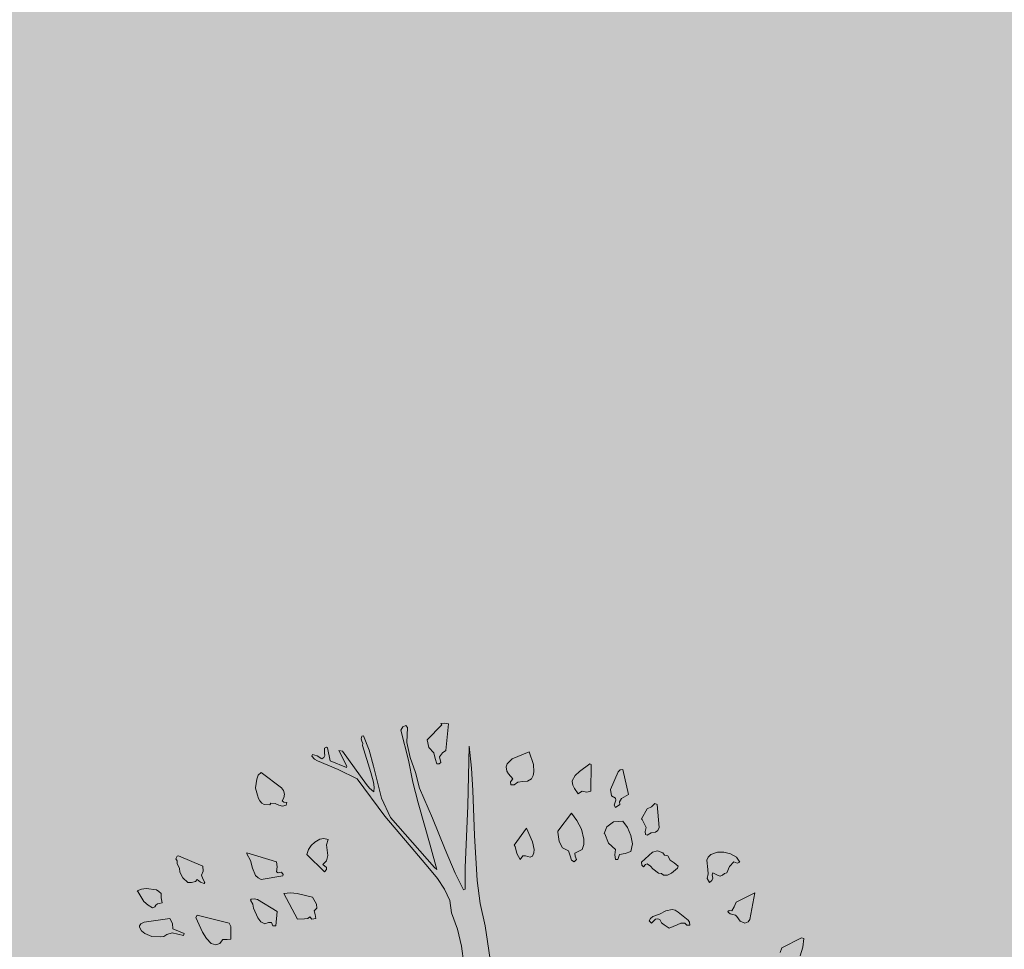
# Model space of a CAD drawing. Units: inches. Extents: x 84 to 1044, y -280 to 906.
# Tile 36 of 105: x 848 to 876, y -93 to -66. Entities that reach past the tile are written whole.
import ezdxf

# ---------------------------------------------------------------- set-up
doc = ezdxf.new("R2010")
doc.units = ezdxf.units.IN
doc.layers.add('L-PLNT', color=114, linetype='Continuous', lineweight=15)
doc.layers.add('L-PLNT-PATT', color=9, linetype='Continuous', lineweight=9, true_color=0xafd9aa)

# ---------------------------------------------------------------- blocks, each defined once
blk = doc.blocks.new('A$C37E508DF')
for p, q in [((0.6329, 1.5111), (0.6367, 1.5175)), ((0.6367, 1.5175), (0.6423, 1.5201)), ((0.6423, 1.5201), (0.6453, 1.5158)), ((0.6826, 1.493), (0.7096, 1.5209)), ((0.7083, 1.5239), (0.7152, 1.5244)), ((0.7096, 1.5209), (0.7083, 1.5239)), ((0.7152, 1.5244), (0.7225, 1.5231)), ((0.7225, 1.5231), (0.7174, 1.4729)), ((0.5583, 1.4948), (0.5596, 1.4995)), ((0.5596, 1.4995), (0.563, 1.5003)), ((0.563, 1.5003), (0.5737, 1.4733)), ((0.6475, 1.4545), (0.6329, 1.5111)), ((0.6453, 1.5158), (0.644, 1.4879)), ((0.5596, 1.4905), (0.5583, 1.4948)), ((0.5613, 1.4862), (0.5596, 1.4905)), ((0.5608, 1.4823), (0.5613, 1.4862)), ((0.5767, 1.4317), (0.5608, 1.4823)), ((0.644, 1.4879), (0.6505, 1.46)), ((0.6852, 1.4785), (0.6826, 1.493)), ((0.7589, 1.3691), (0.7615, 1.481)), ((0.7615, 1.481), (0.7658, 1.4395)), ((0.4657, 1.4622), (0.4669, 1.4652)), ((0.4708, 1.4566), (0.4657, 1.4622)), ((0.4669, 1.4652), (0.4755, 1.463)), ((0.4755, 1.463), (0.4845, 1.4575)), ((0.4884, 1.4596), (0.4905, 1.4635)), ((0.4897, 1.4772), (0.4935, 1.4789)), ((0.4897, 1.4678), (0.4897, 1.4772)), ((0.4905, 1.4635), (0.4897, 1.4678)), ((0.4935, 1.4789), (0.4952, 1.478)), ((0.4952, 1.478), (0.5004, 1.4532)), ((0.5313, 1.4437), (0.5167, 1.4729)), ((0.5167, 1.4729), (0.5231, 1.4716)), ((0.5231, 1.4716), (0.5686, 1.409)), ((0.5737, 1.4733), (0.5814, 1.4437)), ((0.6946, 1.4682), (0.6852, 1.4785)), ((0.6976, 1.4579), (0.6946, 1.4682)), ((0.7109, 1.4682), (0.7053, 1.4609)), ((0.7053, 1.4609), (0.7083, 1.4502)), ((0.7174, 1.4729), (0.7109, 1.4682)), ((0.8421, 1.4575), (0.8739, 1.4703)), ((0.8739, 1.4703), (0.882, 1.4463)), ((0.4764, 1.4532), (0.4708, 1.4566)), ((0.5154, 1.4373), (0.4764, 1.4532)), ((0.4845, 1.4575), (0.4884, 1.4596)), ((0.5004, 1.4532), (0.5308, 1.4412)), ((0.5308, 1.4412), (0.5313, 1.4437)), ((0.5814, 1.4437), (0.5969, 1.3833)), ((0.6552, 1.4137), (0.6475, 1.4545)), ((0.6505, 1.46), (0.6603, 1.4317)), ((0.7002, 1.4476), (0.6976, 1.4579)), ((0.7049, 1.448), (0.7002, 1.4476)), ((0.7083, 1.4502), (0.7049, 1.448)), ((0.831, 1.4424), (0.8323, 1.4476)), ((0.8318, 1.4343), (0.831, 1.4424)), ((0.8323, 1.4476), (0.8357, 1.451)), ((0.8357, 1.451), (0.8421, 1.4575)), ((0.882, 1.4463), (0.8829, 1.433)), ((0.9686, 1.4334), (0.9875, 1.4476)), ((0.9875, 1.4476), (0.9905, 1.4467)), ((0.9905, 1.4467), (0.9896, 1.3966)), ((0.3628, 1.4189), (0.3649, 1.4266)), ((0.3649, 1.4266), (0.3709, 1.4317)), ((0.3709, 1.4317), (0.4086, 1.403)), ((0.551, 1.4197), (0.5154, 1.4373)), ((0.5814, 1.4133), (0.5767, 1.4317)), ((0.6603, 1.4317), (0.668, 1.4021)), ((0.7658, 1.4395), (0.7684, 1.3979)), ((0.8353, 1.4292), (0.8318, 1.4343)), ((0.8434, 1.4197), (0.8353, 1.4292)), ((0.8816, 1.4262), (0.8781, 1.4197)), ((0.8829, 1.433), (0.8816, 1.4262)), ((0.9545, 1.4159), (0.9605, 1.4257)), ((0.9605, 1.4257), (0.9686, 1.4334)), ((1.0269, 1.3996), (1.0411, 1.433)), ((1.0411, 1.433), (1.045, 1.4365)), ((1.045, 1.4365), (1.0497, 1.4369)), ((1.0497, 1.4369), (1.0604, 1.3901)), ((0.3598, 1.403), (0.3628, 1.4189)), ((0.6029, 1.3494), (0.551, 1.4197)), ((0.5686, 1.409), (0.5741, 1.4021)), ((0.5827, 1.4043), (0.5814, 1.4133)), ((0.6655, 1.3743), (0.6552, 1.4137)), ((0.8391, 1.4141), (0.8434, 1.4197)), ((0.8395, 1.4086), (0.8391, 1.4141)), ((0.846, 1.4086), (0.8395, 1.4086)), ((0.8528, 1.4137), (0.846, 1.4086)), ((0.8619, 1.4146), (0.8528, 1.4137)), ((0.8709, 1.4154), (0.8619, 1.4146)), ((0.8781, 1.4197), (0.8709, 1.4154)), ((0.9549, 1.4146), (0.9545, 1.4159)), ((0.9558, 1.4077), (0.9549, 1.4146)), ((0.9592, 1.4017), (0.9558, 1.4077)), ((0.3602, 1.4021), (0.3598, 1.403)), ((0.364, 1.3888), (0.3602, 1.4021)), ((0.3657, 1.3828), (0.364, 1.3888)), ((0.4086, 1.403), (0.4125, 1.3979)), ((0.4125, 1.3979), (0.4142, 1.391)), ((0.4142, 1.391), (0.4134, 1.3837)), ((0.5741, 1.4021), (0.5823, 1.3953)), ((0.5823, 1.3953), (0.5827, 1.4043)), ((0.668, 1.4021), (0.6925, 1.3455)), ((0.7684, 1.3979), (0.771, 1.3134)), ((0.966, 1.3914), (0.9592, 1.4017)), ((0.9703, 1.3944), (0.966, 1.3914)), ((0.9733, 1.3966), (0.9703, 1.3944)), ((0.9819, 1.3944), (0.9733, 1.3966)), ((0.9896, 1.3966), (0.9819, 1.3944)), ((1.0282, 1.3876), (1.0269, 1.3996)), ((1.0359, 1.3833), (1.0282, 1.3876)), ((1.0604, 1.3901), (1.0471, 1.3824)), ((0.3683, 1.3781), (0.3657, 1.3828)), ((0.3718, 1.3738), (0.3683, 1.3781)), ((0.3765, 1.3713), (0.3718, 1.3738)), ((0.3872, 1.3708), (0.3765, 1.3713)), ((0.3885, 1.3738), (0.3872, 1.3708)), ((0.3971, 1.3734), (0.3885, 1.3738)), ((0.4039, 1.3704), (0.3971, 1.3734)), ((0.4108, 1.3683), (0.4039, 1.3704)), ((0.4134, 1.3837), (0.4099, 1.3781)), ((0.4099, 1.3781), (0.4134, 1.376)), ((0.4176, 1.37), (0.4108, 1.3683)), ((0.4134, 1.376), (0.4189, 1.3751)), ((0.4189, 1.3751), (0.4176, 1.37)), ((0.5969, 1.3833), (0.6132, 1.3472)), ((0.6882, 1.2949), (0.6655, 1.3743)), ((0.7538, 1.2529), (0.7589, 1.3691)), ((1.0334, 1.37), (1.0351, 1.376)), ((1.0359, 1.3661), (1.0334, 1.37)), ((1.0351, 1.376), (1.0368, 1.3794)), ((1.0368, 1.3794), (1.0359, 1.3833)), ((1.0441, 1.3717), (1.0359, 1.3661)), ((1.0471, 1.3824), (1.0432, 1.3764)), ((1.0432, 1.3764), (1.0441, 1.3717)), ((1.1033, 1.367), (1.1097, 1.373)), ((1.1097, 1.373), (1.114, 1.3717)), ((1.114, 1.3717), (1.1183, 1.328)), ((0.9274, 1.3215), (0.9532, 1.3554)), ((0.9532, 1.3554), (0.9635, 1.3413)), ((1.0848, 1.3443), (1.0955, 1.3631)), ((1.0955, 1.3631), (1.1033, 1.367)), ((0.6595, 1.2829), (0.6029, 1.3494)), ((0.6132, 1.3472), (0.6959, 1.2529)), ((0.6925, 1.3455), (0.7161, 1.2868)), ((0.9635, 1.3413), (0.9721, 1.325)), ((1.0197, 1.3297), (1.0321, 1.3387)), ((1.0321, 1.3387), (1.0497, 1.3404)), ((1.0497, 1.3404), (1.0587, 1.3284)), ((1.0861, 1.343), (1.0848, 1.3443)), ((1.0938, 1.328), (1.0861, 1.343)), ((0.771, 1.3134), (0.7761, 1.2285)), ((0.846, 1.2949), (0.8687, 1.3271)), ((0.8687, 1.3271), (0.8803, 1.3014)), ((0.9279, 1.3194), (0.9274, 1.3215)), ((0.9305, 1.3018), (0.9279, 1.3194)), ((0.9721, 1.325), (0.9768, 1.3061)), ((1.0149, 1.3172), (1.0171, 1.3232)), ((1.0162, 1.3164), (1.0149, 1.3172)), ((1.0231, 1.2988), (1.0162, 1.3164)), ((1.0171, 1.3232), (1.0197, 1.3297)), ((1.0587, 1.3284), (1.0651, 1.3134)), ((1.0651, 1.3134), (1.0677, 1.2975)), ((1.0917, 1.3207), (1.0938, 1.328)), ((1.0925, 1.3151), (1.0917, 1.3207)), ((1.0955, 1.3138), (1.0925, 1.3151)), ((1.1028, 1.3185), (1.0955, 1.3138)), ((1.111, 1.3194), (1.1028, 1.3185)), ((1.1153, 1.3228), (1.111, 1.3194)), ((1.1183, 1.328), (1.1153, 1.3228)), ((0.4597, 1.2868), (0.4648, 1.2945)), ((0.4648, 1.2945), (0.4717, 1.3009)), ((0.4717, 1.3009), (0.4807, 1.3065)), ((0.4807, 1.3065), (0.4884, 1.3074)), ((0.4884, 1.3074), (0.4965, 1.3057)), ((0.4965, 1.3057), (0.4935, 1.2954)), ((0.4935, 1.2954), (0.4948, 1.2855)), ((0.7002, 1.2495), (0.6882, 1.2949)), ((0.8473, 1.2924), (0.846, 1.2949)), ((0.8803, 1.3014), (0.8833, 1.2872)), ((0.9365, 1.2902), (0.9305, 1.3018)), ((0.9763, 1.2962), (0.9733, 1.2868)), ((0.9768, 1.3061), (0.9763, 1.2962)), ((1.0359, 1.2868), (1.0231, 1.2988)), ((1.0677, 1.2975), (1.0647, 1.2829)), ((0.3439, 1.2804), (0.3992, 1.2636)), ((0.3439, 1.2787), (0.3439, 1.2804)), ((0.3507, 1.2662), (0.3439, 1.2787)), ((0.4562, 1.2774), (0.4597, 1.2868)), ((0.4897, 1.2452), (0.4562, 1.2774)), ((0.4948, 1.2855), (0.4961, 1.2756)), ((0.6865, 1.2508), (0.6595, 1.2829)), ((0.7161, 1.2868), (0.7349, 1.2422)), ((0.8507, 1.2795), (0.8473, 1.2924)), ((0.8567, 1.2679), (0.8507, 1.2795)), ((0.8829, 1.2808), (0.8799, 1.2744)), ((0.8833, 1.2872), (0.8829, 1.2808)), ((0.9476, 1.2842), (0.9365, 1.2902)), ((0.951, 1.2748), (0.9476, 1.2842)), ((0.9733, 1.2868), (0.9596, 1.2799)), ((0.9596, 1.2799), (0.9605, 1.2744)), ((1.0347, 1.2769), (1.0359, 1.2868)), ((1.0359, 1.2679), (1.0347, 1.2769)), ((1.0432, 1.2774), (1.0402, 1.2679)), ((1.0544, 1.2791), (1.0432, 1.2774)), ((1.0647, 1.2829), (1.0544, 1.2791)), ((1.0848, 1.2628), (1.1054, 1.2817)), ((1.1054, 1.2817), (1.1148, 1.2842)), ((1.1148, 1.2842), (1.1247, 1.2804)), ((1.1247, 1.2804), (1.1281, 1.2765)), ((1.1281, 1.2765), (1.1341, 1.2752)), ((1.21, 1.2726), (1.2147, 1.2774)), ((1.2147, 1.2774), (1.2276, 1.2817)), ((1.2276, 1.2817), (1.2392, 1.2817)), ((1.2392, 1.2817), (1.2521, 1.2787)), ((1.2521, 1.2787), (1.2632, 1.2722)), ((0.2101, 1.2696), (0.2127, 1.2744)), ((0.2127, 1.2654), (0.2101, 1.2696)), ((0.2127, 1.2744), (0.2152, 1.2752)), ((0.2127, 1.2602), (0.2127, 1.2654)), ((0.2174, 1.2521), (0.2127, 1.2602)), ((0.2152, 1.2752), (0.2611, 1.2559)), ((0.3546, 1.2516), (0.3507, 1.2662)), ((0.3992, 1.2636), (0.4005, 1.2546)), ((0.4935, 1.2658), (0.4867, 1.2589)), ((0.4867, 1.2589), (0.4935, 1.2529)), ((0.4961, 1.2756), (0.4935, 1.2658)), ((0.8619, 1.2752), (0.8567, 1.2679)), ((0.867, 1.2752), (0.8619, 1.2752)), ((0.8713, 1.2739), (0.867, 1.2752)), ((0.8756, 1.2726), (0.8713, 1.2739)), ((0.8799, 1.2744), (0.8756, 1.2726)), ((0.9532, 1.2666), (0.951, 1.2748)), ((0.9583, 1.2636), (0.9532, 1.2666)), ((0.9626, 1.2679), (0.9583, 1.2636)), ((0.9605, 1.2744), (0.9626, 1.2679)), ((1.0402, 1.2679), (1.0359, 1.2679)), ((1.0852, 1.2576), (1.0848, 1.2628)), ((1.0883, 1.2546), (1.0852, 1.2576)), ((1.0921, 1.2585), (1.0883, 1.2546)), ((1.0955, 1.2602), (1.0921, 1.2585)), ((1.1015, 1.2559), (1.0955, 1.2602)), ((1.1341, 1.2752), (1.1384, 1.2666)), ((1.1384, 1.2666), (1.1461, 1.2619)), ((1.1461, 1.2619), (1.1539, 1.2559)), ((1.2075, 1.2666), (1.21, 1.2726)), ((1.2096, 1.2491), (1.2075, 1.2666)), ((1.2585, 1.2636), (1.2503, 1.2551)), ((1.2645, 1.2615), (1.2585, 1.2636)), ((1.2632, 1.2722), (1.2692, 1.2628)), ((1.2692, 1.2628), (1.2645, 1.2615)), ((0.2182, 1.2443), (0.2174, 1.2521)), ((0.2234, 1.2336), (0.2182, 1.2443)), ((0.262, 1.2465), (0.2586, 1.2388)), ((0.2586, 1.2388), (0.2611, 1.2319)), ((0.2611, 1.2559), (0.262, 1.2465)), ((0.3602, 1.2383), (0.3546, 1.2516)), ((0.4005, 1.2546), (0.3992, 1.2452)), ((0.3992, 1.2452), (0.4026, 1.2431)), ((0.4026, 1.2431), (0.4086, 1.2443)), ((0.4086, 1.2443), (0.4121, 1.2401)), ((0.4121, 1.2401), (0.4112, 1.2375)), ((0.4931, 1.2491), (0.4897, 1.2452)), ((0.4935, 1.2529), (0.4931, 1.2491)), ((0.7015, 1.2323), (0.6865, 1.2508)), ((0.6959, 1.2529), (0.7002, 1.2495)), ((0.7349, 1.2422), (0.7482, 1.216)), ((0.7538, 1.2122), (0.7538, 1.2529)), ((1.1063, 1.2508), (1.1015, 1.2559)), ((1.117, 1.2422), (1.1063, 1.2508)), ((1.1221, 1.2418), (1.117, 1.2422)), ((1.126, 1.2388), (1.1221, 1.2418)), ((1.1337, 1.2388), (1.126, 1.2388)), ((1.141, 1.2422), (1.1337, 1.2388)), ((1.1526, 1.2521), (1.141, 1.2422)), ((1.1539, 1.2559), (1.1526, 1.2521)), ((1.2079, 1.2323), (1.21, 1.2409)), ((1.21, 1.2409), (1.2096, 1.2491)), ((1.2186, 1.2431), (1.2173, 1.2392)), ((1.2173, 1.2392), (1.2186, 1.2332)), ((1.2285, 1.2383), (1.2186, 1.2431)), ((1.2371, 1.2388), (1.2328, 1.2366)), ((1.2405, 1.2418), (1.2371, 1.2388)), ((1.2448, 1.2431), (1.2405, 1.2418)), ((1.2503, 1.2551), (1.2448, 1.2431)), ((0.2328, 1.2251), (0.2234, 1.2336)), ((0.2401, 1.2251), (0.2328, 1.2251)), ((0.2474, 1.2268), (0.2401, 1.2251)), ((0.2504, 1.2306), (0.2474, 1.2268)), ((0.2568, 1.2255), (0.2504, 1.2306)), ((0.2633, 1.2229), (0.2568, 1.2255)), ((0.2611, 1.2319), (0.265, 1.2251)), ((0.265, 1.2251), (0.2633, 1.2229)), ((0.3649, 1.2336), (0.3602, 1.2383)), ((0.3709, 1.2306), (0.3649, 1.2336)), ((0.4112, 1.2375), (0.3709, 1.2306)), ((0.7148, 1.2126), (0.7015, 1.2323)), ((0.7761, 1.2285), (0.7821, 1.1856)), ((1.2126, 1.2251), (1.2079, 1.2323)), ((1.2169, 1.2285), (1.2126, 1.2251)), ((1.2186, 1.2332), (1.2169, 1.2285)), ((1.2328, 1.2366), (1.2285, 1.2383)), ((0.1376, 1.2092), (0.1458, 1.2126)), ((0.1389, 1.2079), (0.1376, 1.2092)), ((0.1505, 1.189), (0.1389, 1.2079)), ((0.1458, 1.2126), (0.1548, 1.2135)), ((0.1548, 1.2135), (0.1741, 1.2109)), ((0.1741, 1.2109), (0.1784, 1.2083)), ((0.1784, 1.2083), (0.1831, 1.204)), ((0.1831, 1.204), (0.1831, 1.1959)), ((0.4134, 1.204), (0.4258, 1.2058)), ((0.4391, 1.156), (0.4134, 1.204)), ((0.4258, 1.2058), (0.4382, 1.2045)), ((0.4382, 1.2045), (0.4669, 1.1972)), ((0.7246, 1.1908), (0.7148, 1.2126)), ((0.7482, 1.216), (0.7508, 1.2109)), ((0.7508, 1.2109), (0.7538, 1.2122)), ((1.2628, 1.1882), (1.2975, 1.2053)), ((1.2975, 1.2053), (1.2885, 1.1556)), ((0.1582, 1.1822), (0.1505, 1.189)), ((0.1758, 1.1847), (0.1728, 1.1826)), ((0.1788, 1.1852), (0.1758, 1.1847)), ((0.1848, 1.1865), (0.1788, 1.1852)), ((0.1831, 1.1959), (0.1848, 1.1865)), ((0.3507, 1.1916), (0.352, 1.1933)), ((0.355, 1.1839), (0.3507, 1.1916)), ((0.352, 1.1933), (0.3576, 1.1942)), ((0.3563, 1.177), (0.355, 1.1839)), ((0.3576, 1.1942), (0.364, 1.1929)), ((0.364, 1.1929), (0.4005, 1.1702)), ((0.4669, 1.1972), (0.4747, 1.1843)), ((0.4747, 1.1843), (0.4751, 1.177)), ((0.7281, 1.168), (0.7246, 1.1908)), ((0.7821, 1.1856), (0.7911, 1.1436)), ((1.2589, 1.1792), (1.2628, 1.1882)), ((0.1668, 1.1775), (0.1582, 1.1822)), ((0.1711, 1.1792), (0.1668, 1.1775)), ((0.1728, 1.1826), (0.1711, 1.1792)), ((0.3645, 1.1586), (0.3563, 1.177)), ((0.4005, 1.1702), (0.3979, 1.1436)), ((0.4751, 1.177), (0.47, 1.1714)), ((0.47, 1.1714), (0.4721, 1.1646)), ((0.7396, 1.1371), (0.7281, 1.168)), ((1.1063, 1.1612), (1.1187, 1.1655)), ((1.1187, 1.1655), (1.1307, 1.1714)), ((1.1307, 1.1714), (1.1423, 1.1744)), ((1.1423, 1.1744), (1.1483, 1.1732)), ((1.1483, 1.1732), (1.1539, 1.1693)), ((1.1539, 1.1693), (1.1727, 1.1543)), ((1.2469, 1.1702), (1.2495, 1.1723)), ((1.2478, 1.1693), (1.2469, 1.1702)), ((1.2516, 1.1659), (1.2478, 1.1693)), ((1.2495, 1.1723), (1.2546, 1.1719)), ((1.2563, 1.1646), (1.2516, 1.1659)), ((1.2546, 1.1719), (1.2589, 1.1792)), ((0.1419, 1.1436), (0.1449, 1.1474)), ((0.1449, 1.1474), (0.1509, 1.1504)), ((0.1509, 1.1504), (0.1994, 1.1573)), ((0.1994, 1.1573), (0.2041, 1.1479)), ((0.2041, 1.1479), (0.2045, 1.138)), ((0.2478, 1.1594), (0.2504, 1.1637)), ((0.2607, 1.1316), (0.2478, 1.1594)), ((0.2504, 1.1637), (0.3104, 1.1487)), ((0.3104, 1.1487), (0.3134, 1.1423)), ((0.37, 1.1509), (0.3645, 1.1586)), ((0.3778, 1.1474), (0.37, 1.1509)), ((0.3842, 1.15), (0.3778, 1.1474)), ((0.3898, 1.15), (0.3842, 1.15)), ((0.3923, 1.1436), (0.3898, 1.15)), ((0.4519, 1.1564), (0.4391, 1.156)), ((0.458, 1.1573), (0.4519, 1.1564)), ((0.4622, 1.1607), (0.458, 1.1573)), ((0.4657, 1.156), (0.4622, 1.1607)), ((0.473, 1.1573), (0.4657, 1.156)), ((0.4721, 1.1646), (0.473, 1.1573)), ((1.099, 1.153), (1.102, 1.1573)), ((1.1033, 1.1487), (1.099, 1.153)), ((1.102, 1.1573), (1.1063, 1.1612)), ((1.111, 1.156), (1.1033, 1.1487)), ((1.1153, 1.1564), (1.111, 1.156)), ((1.1191, 1.1556), (1.1153, 1.1564)), ((1.1226, 1.1492), (1.1191, 1.1556)), ((1.1273, 1.1453), (1.1226, 1.1492)), ((1.1586, 1.1483), (1.1517, 1.1453)), ((1.1663, 1.1487), (1.1586, 1.1483)), ((1.1697, 1.1449), (1.1663, 1.1487)), ((1.1727, 1.1543), (1.1749, 1.1504)), ((1.1749, 1.1504), (1.1757, 1.1449)), ((1.2611, 1.1637), (1.2563, 1.1646)), ((1.2641, 1.1612), (1.2611, 1.1637)), ((1.2701, 1.1522), (1.2641, 1.1612)), ((1.2791, 1.1487), (1.2701, 1.1522)), ((1.2851, 1.1509), (1.2791, 1.1487)), ((1.2885, 1.1556), (1.2851, 1.1509)), ((0.1419, 1.141), (0.1419, 1.1436)), ((0.1462, 1.1342), (0.1419, 1.141)), ((0.1522, 1.1294), (0.1462, 1.1342)), ((0.1655, 1.1234), (0.1522, 1.1294)), ((0.2032, 1.1303), (0.1938, 1.1273)), ((0.2247, 1.1251), (0.2032, 1.1303)), ((0.2045, 1.138), (0.226, 1.129)), ((0.226, 1.129), (0.2247, 1.1251)), ((0.268, 1.1196), (0.2607, 1.1316)), ((0.3134, 1.1423), (0.3139, 1.1346)), ((0.3139, 1.1346), (0.3134, 1.1183)), ((0.3979, 1.1436), (0.3923, 1.1436)), ((0.7469, 1.1054), (0.7396, 1.1371)), ((0.7911, 1.1436), (0.8027, 1.0677)), ((1.1367, 1.1393), (1.1273, 1.1453)), ((1.1517, 1.1453), (1.1367, 1.1393)), ((1.1757, 1.1449), (1.1697, 1.1449)), ((0.181, 1.1226), (0.1655, 1.1234)), ((0.1878, 1.1234), (0.181, 1.1226)), ((0.1938, 1.1273), (0.1878, 1.1234)), ((0.277, 1.1101), (0.268, 1.1196)), ((0.2856, 1.108), (0.277, 1.1101)), ((0.2933, 1.1101), (0.2856, 1.108)), ((0.2959, 1.1144), (0.2933, 1.1101)), ((0.2984, 1.1179), (0.2959, 1.1144)), ((0.3066, 1.1179), (0.2984, 1.1179)), ((0.3134, 1.1183), (0.3066, 1.1179)), ((1.3485, 1.102), (1.385, 1.1209)), ((1.385, 1.1209), (1.3897, 1.1196)), ((1.3897, 1.1196), (1.3875, 1.1037)), ((0.7512, 1.0728), (0.7469, 1.1054)), ((1.3455, 1.0934), (1.3485, 1.102)), ((1.3875, 1.1037), (1.3828, 1.087))]:
    blk.add_line(p, q)

msp = doc.modelspace()

# ---------------------------------------------------------------- hatches: boundary and pattern name
at = {"layer": 'L-PLNT-PATT', "transparency": 33554597}
h = msp.add_hatch(color=256, dxfattribs=at)
h.dxf.hatch_style = 1
h.paths.add_polyline_path([(791.074, 31.12), (791.074, 91.12), (743.074, 91.12), (674.074, 91.12), (674.074, 31.12), (650.074, 31.12), (650.074, -112.88), (983.074, -112.88), (983.074, -64.88), (791.074, -64.88)])

# ---------------------------------------------------------------- block references
at = {"layer": 'L-PLNT', "xscale": 15.19586232982809, "yscale": 15.19586232982809, "zscale": 15.19586232982809}
msp.add_blockref('A$C37E508DF', (849.112, -109.703, 0), dxfattribs=at)

doc.saveas('drawing.dxf')
